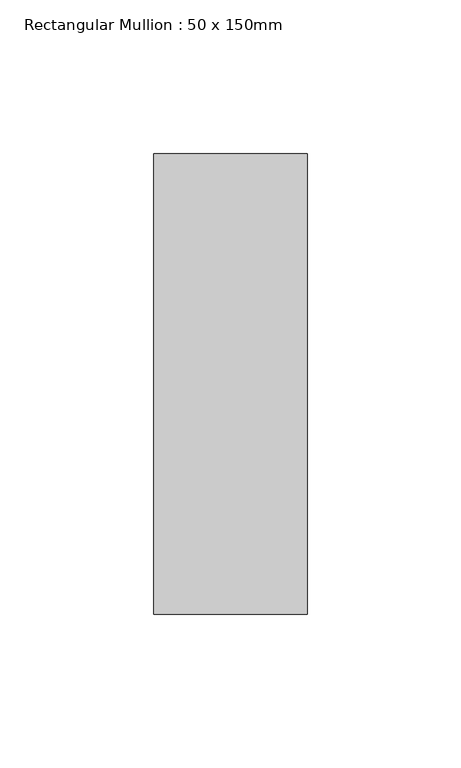
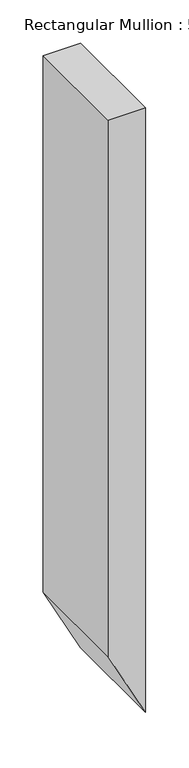
"""IFC4 building model written with IfcOpenShell, lengths in millimetres: member geometry, Rectangular Mullion : 50 x 150mm."""

from ifc_helpers import new_model, si_unit, frame, origin, place, context, project, spatial, polyline, outline, extrude, source, transform, mapped, element, save


def rectangular_mullion_50_x_150mm_5b89cbb4(model_context):
    return source(origin(), model_context, "Body", "SweptSolid", [
        extrude(outline(polyline([(0.0, 0.0), (0.0, -50.0), (-756.0404197, -50.0), (-852.089526, 0.0), (0.0, 0.0)])), frame((0.0, -75.0, 0.0), z_axis=(0.0, 1.0, 0.0), x_axis=(0.0, 0.0, 1.0)), (0.0, 0.0, 1.0), 150.0),
    ])


if __name__ == "__main__":
    model = new_model("IFC4")
    model_context = context("Model", 3, world=origin())
    ifc_project = project(units=[si_unit("LENGTHUNIT", "METRE", prefix="MILLI")], contexts=[model_context])
    site = spatial("IfcSite", under=ifc_project)
    building = spatial("IfcBuilding", under=site)
    placement = place(None, origin())
    rectangular_mullion_50_x_150mm_shape = rectangular_mullion_50_x_150mm_5b89cbb4(model_context)
    element("IfcMember", 1, ObjectType="Rectangular Mullion : 50 x 150mm", at=placement, inside=building, context=model_context, shape_type="MappedRepresentation", body=[
        mapped(rectangular_mullion_50_x_150mm_shape, transform((0.0, 0.0, 0.0), x_axis=(1.0, 0.0, 0.0), y_axis=(0.0, 1.0, 0.0), z_axis=(0.0, 0.0, 1.0))),
    ])
    save(model, "model.ifc")

# Revit data of these elements
# Type "Rectangular Mullion : 50 x 150mm"
#   built-in parameter 1007304 = 0.492126 (stored number, unit not read)
#   built-in parameter 1007301 = 0.082021 (stored number, unit not read)
#   built-in parameter 1007300 = 0.082021 (stored number, unit not read)
# Element 1 (IfcMember, "Rectangular Mullion : 50 x 150mm")
#   Materials on its faces: "Aluminium"
# Materials
#   "Aluminium": class "Metal", colour RGB 247 247 247, transparency 0, Description = "Aluminium 6061", Cost = 0
